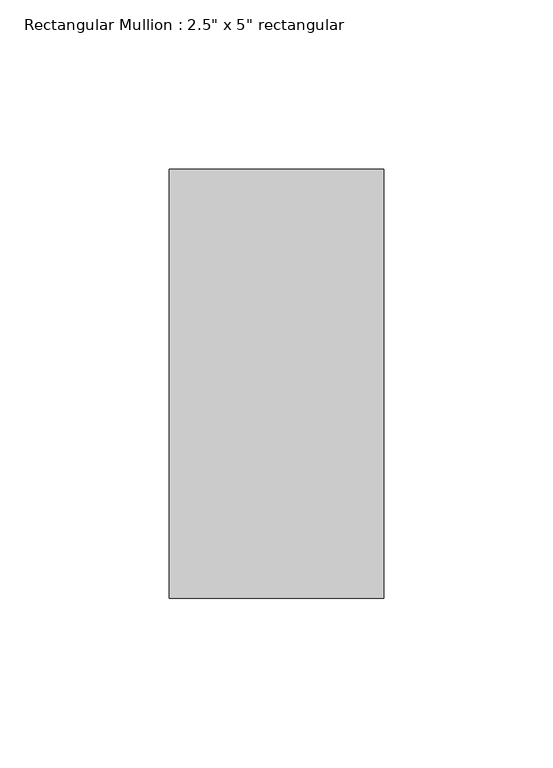
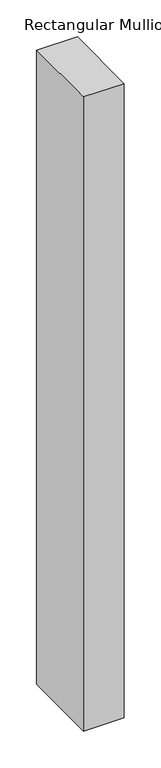
"""IFC4 building model written with IfcOpenShell, lengths in millimetres: member geometry."""

from ifc_helpers import new_model, si_unit, frame, origin, place, context, project, spatial, polyline, outline, extrude, source, transform, mapped, element, save


def member_697f972d(model_context):
    return source(origin(), model_context, "Body", "SweptSolid", [
        extrude(outline(polyline([(31.75, 63.5), (31.75, -63.5), (-31.75, -63.5), (-31.75, 63.5), (31.75, 63.5)])), frame((0.0, 0.0, -1047.75), z_axis=(0.0, 0.0, 1.0), x_axis=(1.0, 0.0, 0.0)), (0.0, 0.0, 1.0), 1047.75),
    ])


if __name__ == "__main__":
    model = new_model("IFC4")
    model_context = context("Model", 3, world=origin())
    ifc_project = project(units=[si_unit("LENGTHUNIT", "METRE", prefix="MILLI")], contexts=[model_context])
    site = spatial("IfcSite", under=ifc_project)
    building = spatial("IfcBuilding", under=site)
    placement = place(None, origin())
    member_shape = member_697f972d(model_context)
    element("IfcMember", 1, ObjectType="Rectangular Mullion : 2.5\" x 5\" rectangular", at=placement, inside=building, context=model_context, shape_type="MappedRepresentation", body=[
        mapped(member_shape, transform((0.0, 0.0, 0.0), x_axis=(1.0, 0.0, 0.0), y_axis=(0.0, 1.0, 0.0), z_axis=(0.0, 0.0, 1.0))),
    ])
    save(model, "model.ifc")

# Revit data of these elements
# Type "Rectangular Mullion : 2.5\" x 5\" rectangular"
#   built-in parameter 1007304 = 0.416667 (stored number, unit not read)
#   built-in parameter 1007301 = 0.104167 (stored number, unit not read)
#   built-in parameter 1007300 = 0.104167 (stored number, unit not read)
# Element 1 (IfcMember, "Rectangular Mullion : 2.5\" x 5\" rectangular")
#   Materials on its faces: "Aluminum"
# Materials
#   "Aluminum": class "Metal", colour RGB 247 247 247, transparency 0, Description = "Aluminum 6061", Cost = 0
